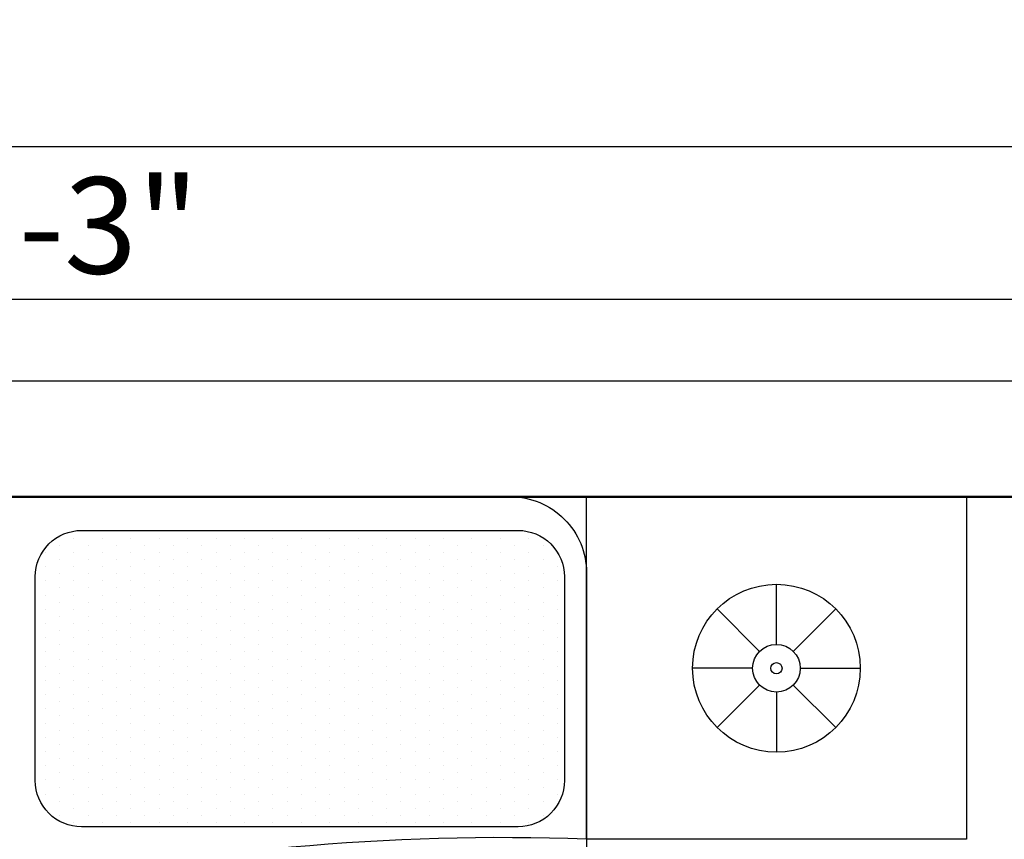
# Model space of a CAD drawing. Units: inches. Extents: x 3064 to 19385, y 846 to 15425.
# Tile 63 of 108: x 6281 to 6332, y 1964 to 2007. Entities that reach past the tile are written whole.
import ezdxf

# ---------------------------------------------------------------- set-up
doc = ezdxf.new("R2010")
doc.units = ezdxf.units.IN
for name, color, linetype, lineweight in [('A-ANNO-DIMS', 2, 'Continuous', 18), ('A-FLOR-FIXT', 9, 'Continuous', 18), ('A-WALL', 7, 'Continuous', 50), ('C-PROP', 6, 'Continuous', 25)]:
    doc.layers.add(name, color=color, linetype=linetype, lineweight=lineweight)
doc.layers.add('BLOCK', color=6, linetype='Continuous')
doc.styles.get("Standard").update_dxf_attribs({"font": 'arial.ttf'})
doc.dimstyles.new('ISO-25', dxfattribs={"dimtxt": 9, "dimasz": 2.5, "dimexe": 1.25, "dimexo": 0.625, "dimtad": 1, "dimdec": 1, "dimlunit": 3, "dimtxsty": 'Standard', "dimcen": 2.5, "dimadec": 0, "dimazin": 0, "dimtfac": 1, "dimtdec": 1, "dimtmove": 0, "dimatfit": 3, "dimfxl": 1, "dimarcsym": 0})

# ---------------------------------------------------------------- blocks, each defined once
blk = doc.blocks.new('*X7')
at = {"color": 0}
for p, q in [((273.75, 456.9375), (273.75, 456.9375)), ((273.9375, 457.03125), (273.9375, 457.03125)), ((274.125, 456.9375), (274.125, 456.9375)), ((274.3125, 457.03125), (274.3125, 457.03125)), ((274.5, 456.9375), (274.5, 456.9375)), ((274.6875, 457.03125), (274.6875, 457.03125)), ((274.875, 456.9375), (274.875, 456.9375)), ((275.0625, 457.03125), (275.0625, 457.03125)), ((275.25, 456.9375), (275.25, 456.9375)), ((275.4375, 457.03125), (275.4375, 457.03125)), ((275.625, 456.9375), (275.625, 456.9375)), ((275.8125, 457.03125), (275.8125, 457.03125)), ((276, 456.9375), (276, 456.9375)), ((276.1875, 457.03125), (276.1875, 457.03125)), ((276.375, 456.9375), (276.375, 456.9375)), ((276.5625, 457.03125), (276.5625, 457.03125)), ((276.75, 456.9375), (276.75, 456.9375)), ((276.9375, 457.03125), (276.9375, 457.03125)), ((277.125, 456.9375), (277.125, 456.9375)), ((277.3125, 457.03125), (277.3125, 457.03125)), ((277.5, 456.9375), (277.5, 456.9375)), ((277.6875, 457.03125), (277.6875, 457.03125)), ((277.875, 456.9375), (277.875, 456.9375)), ((278.0625, 457.03125), (278.0625, 457.03125)), ((278.25, 456.9375), (278.25, 456.9375)), ((278.4375, 457.03125), (278.4375, 457.03125)), ((278.625, 456.9375), (278.625, 456.9375)), ((278.8125, 457.03125), (278.8125, 457.03125)), ((279, 456.9375), (279, 456.9375)), ((279.1875, 457.03125), (279.1875, 457.03125)), ((279.375, 456.9375), (279.375, 456.9375)), ((279.5625, 457.03125), (279.5625, 457.03125)), ((279.75, 456.9375), (279.75, 456.9375)), ((273.5625, 456.84375), (273.5625, 456.84375)), ((273.9375, 456.84375), (273.9375, 456.84375)), ((274.3125, 456.84375), (274.3125, 456.84375)), ((274.6875, 456.84375), (274.6875, 456.84375)), ((275.0625, 456.84375), (275.0625, 456.84375)), ((275.4375, 456.84375), (275.4375, 456.84375)), ((275.8125, 456.84375), (275.8125, 456.84375)), ((276.1875, 456.84375), (276.1875, 456.84375)), ((276.5625, 456.84375), (276.5625, 456.84375)), ((276.9375, 456.84375), (276.9375, 456.84375)), ((277.3125, 456.84375), (277.3125, 456.84375)), ((277.6875, 456.84375), (277.6875, 456.84375)), ((278.0625, 456.84375), (278.0625, 456.84375)), ((278.4375, 456.84375), (278.4375, 456.84375)), ((278.8125, 456.84375), (278.8125, 456.84375)), ((279.1875, 456.84375), (279.1875, 456.84375)), ((279.5625, 456.84375), (279.5625, 456.84375)), ((279.9375, 456.84375), (279.9375, 456.84375)), ((273.375, 456.75), (273.375, 456.75)), ((273.5625, 456.65625), (273.5625, 456.65625)), ((273.75, 456.75), (273.75, 456.75)), ((273.9375, 456.65625), (273.9375, 456.65625)), ((274.125, 456.75), (274.125, 456.75)), ((274.3125, 456.65625), (274.3125, 456.65625)), ((274.5, 456.75), (274.5, 456.75)), ((274.6875, 456.65625), (274.6875, 456.65625)), ((274.875, 456.75), (274.875, 456.75)), ((275.0625, 456.65625), (275.0625, 456.65625)), ((275.25, 456.75), (275.25, 456.75)), ((275.4375, 456.65625), (275.4375, 456.65625)), ((275.625, 456.75), (275.625, 456.75)), ((275.8125, 456.65625), (275.8125, 456.65625)), ((276, 456.75), (276, 456.75)), ((276.1875, 456.65625), (276.1875, 456.65625)), ((276.375, 456.75), (276.375, 456.75)), ((276.5625, 456.65625), (276.5625, 456.65625)), ((276.75, 456.75), (276.75, 456.75)), ((276.9375, 456.65625), (276.9375, 456.65625)), ((277.125, 456.75), (277.125, 456.75)), ((277.3125, 456.65625), (277.3125, 456.65625)), ((277.5, 456.75), (277.5, 456.75)), ((277.6875, 456.65625), (277.6875, 456.65625)), ((277.875, 456.75), (277.875, 456.75)), ((278.0625, 456.65625), (278.0625, 456.65625)), ((278.25, 456.75), (278.25, 456.75)), ((278.4375, 456.65625), (278.4375, 456.65625)), ((278.625, 456.75), (278.625, 456.75)), ((278.8125, 456.65625), (278.8125, 456.65625)), ((279, 456.75), (279, 456.75)), ((279.1875, 456.65625), (279.1875, 456.65625)), ((279.375, 456.75), (279.375, 456.75)), ((279.5625, 456.65625), (279.5625, 456.65625)), ((279.75, 456.75), (279.75, 456.75)), ((279.9375, 456.65625), (279.9375, 456.65625)), ((280.125, 456.75), (280.125, 456.75)), ((273.375, 456.5625), (273.375, 456.5625)), ((273.75, 456.5625), (273.75, 456.5625)), ((274.125, 456.5625), (274.125, 456.5625)), ((274.5, 456.5625), (274.5, 456.5625)), ((274.875, 456.5625), (274.875, 456.5625)), ((275.25, 456.5625), (275.25, 456.5625)), ((275.625, 456.5625), (275.625, 456.5625)), ((276, 456.5625), (276, 456.5625)), ((276.375, 456.5625), (276.375, 456.5625)), ((276.75, 456.5625), (276.75, 456.5625)), ((277.125, 456.5625), (277.125, 456.5625)), ((277.5, 456.5625), (277.5, 456.5625)), ((277.875, 456.5625), (277.875, 456.5625)), ((278.25, 456.5625), (278.25, 456.5625)), ((278.625, 456.5625), (278.625, 456.5625)), ((279, 456.5625), (279, 456.5625)), ((279.375, 456.5625), (279.375, 456.5625)), ((279.75, 456.5625), (279.75, 456.5625)), ((280.125, 456.5625), (280.125, 456.5625)), ((273.5625, 456.46875), (273.5625, 456.46875)), ((273.9375, 456.46875), (273.9375, 456.46875)), ((274.3125, 456.46875), (274.3125, 456.46875)), ((274.6875, 456.46875), (274.6875, 456.46875)), ((275.0625, 456.46875), (275.0625, 456.46875)), ((275.4375, 456.46875), (275.4375, 456.46875)), ((275.8125, 456.46875), (275.8125, 456.46875)), ((276.1875, 456.46875), (276.1875, 456.46875)), ((276.5625, 456.46875), (276.5625, 456.46875)), ((276.9375, 456.46875), (276.9375, 456.46875)), ((277.3125, 456.46875), (277.3125, 456.46875)), ((277.6875, 456.46875), (277.6875, 456.46875)), ((278.0625, 456.46875), (278.0625, 456.46875)), ((278.4375, 456.46875), (278.4375, 456.46875)), ((278.8125, 456.46875), (278.8125, 456.46875)), ((279.1875, 456.46875), (279.1875, 456.46875)), ((279.5625, 456.46875), (279.5625, 456.46875)), ((279.9375, 456.46875), (279.9375, 456.46875)), ((273.375, 456.375), (273.375, 456.375)), ((273.5625, 456.28125), (273.5625, 456.28125)), ((273.75, 456.375), (273.75, 456.375)), ((273.9375, 456.28125), (273.9375, 456.28125)), ((274.125, 456.375), (274.125, 456.375)), ((274.3125, 456.28125), (274.3125, 456.28125)), ((274.5, 456.375), (274.5, 456.375)), ((274.6875, 456.28125), (274.6875, 456.28125)), ((274.875, 456.375), (274.875, 456.375)), ((275.0625, 456.28125), (275.0625, 456.28125)), ((275.25, 456.375), (275.25, 456.375)), ((275.4375, 456.28125), (275.4375, 456.28125)), ((275.625, 456.375), (275.625, 456.375)), ((275.8125, 456.28125), (275.8125, 456.28125)), ((276, 456.375), (276, 456.375)), ((276.1875, 456.28125), (276.1875, 456.28125)), ((276.375, 456.375), (276.375, 456.375)), ((276.5625, 456.28125), (276.5625, 456.28125)), ((276.75, 456.375), (276.75, 456.375)), ((276.9375, 456.28125), (276.9375, 456.28125)), ((277.125, 456.375), (277.125, 456.375)), ((277.3125, 456.28125), (277.3125, 456.28125)), ((277.5, 456.375), (277.5, 456.375)), ((277.6875, 456.28125), (277.6875, 456.28125)), ((277.875, 456.375), (277.875, 456.375)), ((278.0625, 456.28125), (278.0625, 456.28125)), ((278.25, 456.375), (278.25, 456.375)), ((278.4375, 456.28125), (278.4375, 456.28125)), ((278.625, 456.375), (278.625, 456.375)), ((278.8125, 456.28125), (278.8125, 456.28125)), ((279, 456.375), (279, 456.375)), ((279.1875, 456.28125), (279.1875, 456.28125)), ((279.375, 456.375), (279.375, 456.375)), ((279.5625, 456.28125), (279.5625, 456.28125)), ((279.75, 456.375), (279.75, 456.375)), ((279.9375, 456.28125), (279.9375, 456.28125)), ((280.125, 456.375), (280.125, 456.375)), ((273.375, 456.1875), (273.375, 456.1875)), ((273.75, 456.1875), (273.75, 456.1875)), ((274.125, 456.1875), (274.125, 456.1875)), ((274.5, 456.1875), (274.5, 456.1875)), ((274.875, 456.1875), (274.875, 456.1875)), ((275.25, 456.1875), (275.25, 456.1875)), ((275.625, 456.1875), (275.625, 456.1875)), ((276, 456.1875), (276, 456.1875)), ((276.375, 456.1875), (276.375, 456.1875)), ((276.75, 456.1875), (276.75, 456.1875)), ((277.125, 456.1875), (277.125, 456.1875)), ((277.5, 456.1875), (277.5, 456.1875)), ((277.875, 456.1875), (277.875, 456.1875)), ((278.25, 456.1875), (278.25, 456.1875)), ((278.625, 456.1875), (278.625, 456.1875)), ((279, 456.1875), (279, 456.1875)), ((279.375, 456.1875), (279.375, 456.1875)), ((279.75, 456.1875), (279.75, 456.1875)), ((280.125, 456.1875), (280.125, 456.1875)), ((273.375, 456), (273.375, 456)), ((273.5625, 456.09375), (273.5625, 456.09375)), ((273.75, 456), (273.75, 456)), ((273.9375, 456.09375), (273.9375, 456.09375)), ((274.125, 456), (274.125, 456)), ((274.3125, 456.09375), (274.3125, 456.09375)), ((274.5, 456), (274.5, 456)), ((274.6875, 456.09375), (274.6875, 456.09375)), ((274.875, 456), (274.875, 456)), ((275.0625, 456.09375), (275.0625, 456.09375)), ((275.25, 456), (275.25, 456)), ((275.4375, 456.09375), (275.4375, 456.09375)), ((275.625, 456), (275.625, 456)), ((275.8125, 456.09375), (275.8125, 456.09375)), ((276, 456), (276, 456)), ((276.1875, 456.09375), (276.1875, 456.09375)), ((276.375, 456), (276.375, 456)), ((276.5625, 456.09375), (276.5625, 456.09375)), ((276.75, 456), (276.75, 456)), ((276.9375, 456.09375), (276.9375, 456.09375)), ((277.125, 456), (277.125, 456)), ((277.3125, 456.09375), (277.3125, 456.09375)), ((277.5, 456), (277.5, 456)), ((277.6875, 456.09375), (277.6875, 456.09375)), ((277.875, 456), (277.875, 456)), ((278.0625, 456.09375), (278.0625, 456.09375)), ((278.25, 456), (278.25, 456)), ((278.4375, 456.09375), (278.4375, 456.09375)), ((278.625, 456), (278.625, 456)), ((278.8125, 456.09375), (278.8125, 456.09375)), ((279, 456), (279, 456)), ((279.1875, 456.09375), (279.1875, 456.09375)), ((279.375, 456), (279.375, 456)), ((279.5625, 456.09375), (279.5625, 456.09375)), ((279.75, 456), (279.75, 456)), ((279.9375, 456.09375), (279.9375, 456.09375)), ((280.125, 456), (280.125, 456)), ((273.5625, 455.90625), (273.5625, 455.90625)), ((273.9375, 455.90625), (273.9375, 455.90625)), ((274.3125, 455.90625), (274.3125, 455.90625)), ((274.6875, 455.90625), (274.6875, 455.90625)), ((275.0625, 455.90625), (275.0625, 455.90625)), ((275.4375, 455.90625), (275.4375, 455.90625)), ((275.8125, 455.90625), (275.8125, 455.90625)), ((276.1875, 455.90625), (276.1875, 455.90625)), ((276.5625, 455.90625), (276.5625, 455.90625)), ((276.9375, 455.90625), (276.9375, 455.90625)), ((277.3125, 455.90625), (277.3125, 455.90625)), ((277.6875, 455.90625), (277.6875, 455.90625)), ((278.0625, 455.90625), (278.0625, 455.90625)), ((278.4375, 455.90625), (278.4375, 455.90625)), ((278.8125, 455.90625), (278.8125, 455.90625)), ((279.1875, 455.90625), (279.1875, 455.90625)), ((279.5625, 455.90625), (279.5625, 455.90625)), ((279.9375, 455.90625), (279.9375, 455.90625)), ((273.375, 455.8125), (273.375, 455.8125)), ((273.75, 455.8125), (273.75, 455.8125)), ((274.125, 455.8125), (274.125, 455.8125)), ((274.5, 455.8125), (274.5, 455.8125)), ((274.875, 455.8125), (274.875, 455.8125)), ((275.25, 455.8125), (275.25, 455.8125)), ((275.625, 455.8125), (275.625, 455.8125)), ((276, 455.8125), (276, 455.8125)), ((276.375, 455.8125), (276.375, 455.8125)), ((276.75, 455.8125), (276.75, 455.8125)), ((277.125, 455.8125), (277.125, 455.8125)), ((277.5, 455.8125), (277.5, 455.8125)), ((277.875, 455.8125), (277.875, 455.8125)), ((278.25, 455.8125), (278.25, 455.8125)), ((278.625, 455.8125), (278.625, 455.8125)), ((279, 455.8125), (279, 455.8125)), ((279.375, 455.8125), (279.375, 455.8125)), ((279.75, 455.8125), (279.75, 455.8125)), ((280.125, 455.8125), (280.125, 455.8125)), ((273.375, 455.625), (273.375, 455.625)), ((273.5625, 455.71875), (273.5625, 455.71875)), ((273.75, 455.625), (273.75, 455.625)), ((273.9375, 455.71875), (273.9375, 455.71875)), ((274.125, 455.625), (274.125, 455.625)), ((274.3125, 455.71875), (274.3125, 455.71875)), ((274.5, 455.625), (274.5, 455.625)), ((274.6875, 455.71875), (274.6875, 455.71875)), ((274.875, 455.625), (274.875, 455.625)), ((275.0625, 455.71875), (275.0625, 455.71875)), ((275.25, 455.625), (275.25, 455.625)), ((275.4375, 455.71875), (275.4375, 455.71875)), ((275.625, 455.625), (275.625, 455.625)), ((275.8125, 455.71875), (275.8125, 455.71875)), ((276, 455.625), (276, 455.625)), ((276.1875, 455.71875), (276.1875, 455.71875)), ((276.375, 455.625), (276.375, 455.625)), ((276.5625, 455.71875), (276.5625, 455.71875)), ((276.75, 455.625), (276.75, 455.625)), ((276.9375, 455.71875), (276.9375, 455.71875)), ((277.125, 455.625), (277.125, 455.625)), ((277.3125, 455.71875), (277.3125, 455.71875)), ((277.5, 455.625), (277.5, 455.625)), ((277.6875, 455.71875), (277.6875, 455.71875)), ((277.875, 455.625), (277.875, 455.625)), ((278.0625, 455.71875), (278.0625, 455.71875)), ((278.25, 455.625), (278.25, 455.625)), ((278.4375, 455.71875), (278.4375, 455.71875)), ((278.625, 455.625), (278.625, 455.625)), ((278.8125, 455.71875), (278.8125, 455.71875)), ((279, 455.625), (279, 455.625)), ((279.1875, 455.71875), (279.1875, 455.71875)), ((279.375, 455.625), (279.375, 455.625)), ((279.5625, 455.71875), (279.5625, 455.71875)), ((279.75, 455.625), (279.75, 455.625)), ((279.9375, 455.71875), (279.9375, 455.71875)), ((280.125, 455.625), (280.125, 455.625)), ((273.5625, 455.53125), (273.5625, 455.53125)), ((273.9375, 455.53125), (273.9375, 455.53125)), ((274.3125, 455.53125), (274.3125, 455.53125)), ((274.6875, 455.53125), (274.6875, 455.53125)), ((275.0625, 455.53125), (275.0625, 455.53125)), ((275.4375, 455.53125), (275.4375, 455.53125)), ((275.8125, 455.53125), (275.8125, 455.53125)), ((276.1875, 455.53125), (276.1875, 455.53125)), ((276.5625, 455.53125), (276.5625, 455.53125)), ((276.9375, 455.53125), (276.9375, 455.53125)), ((277.3125, 455.53125), (277.3125, 455.53125)), ((277.6875, 455.53125), (277.6875, 455.53125)), ((278.0625, 455.53125), (278.0625, 455.53125)), ((278.4375, 455.53125), (278.4375, 455.53125)), ((278.8125, 455.53125), (278.8125, 455.53125)), ((279.1875, 455.53125), (279.1875, 455.53125)), ((279.5625, 455.53125), (279.5625, 455.53125)), ((279.9375, 455.53125), (279.9375, 455.53125)), ((273.375, 455.4375), (273.375, 455.4375)), ((273.75, 455.4375), (273.75, 455.4375)), ((274.125, 455.4375), (274.125, 455.4375)), ((274.5, 455.4375), (274.5, 455.4375)), ((274.875, 455.4375), (274.875, 455.4375)), ((275.25, 455.4375), (275.25, 455.4375)), ((275.625, 455.4375), (275.625, 455.4375)), ((276, 455.4375), (276, 455.4375)), ((276.375, 455.4375), (276.375, 455.4375)), ((276.75, 455.4375), (276.75, 455.4375)), ((277.125, 455.4375), (277.125, 455.4375)), ((277.5, 455.4375), (277.5, 455.4375)), ((277.875, 455.4375), (277.875, 455.4375)), ((278.25, 455.4375), (278.25, 455.4375)), ((278.625, 455.4375), (278.625, 455.4375)), ((279, 455.4375), (279, 455.4375)), ((279.375, 455.4375), (279.375, 455.4375)), ((279.75, 455.4375), (279.75, 455.4375)), ((280.125, 455.4375), (280.125, 455.4375)), ((273.375, 455.25), (273.375, 455.25)), ((273.5625, 455.34375), (273.5625, 455.34375)), ((273.75, 455.25), (273.75, 455.25)), ((273.9375, 455.34375), (273.9375, 455.34375)), ((274.125, 455.25), (274.125, 455.25)), ((274.3125, 455.34375), (274.3125, 455.34375)), ((274.5, 455.25), (274.5, 455.25)), ((274.6875, 455.34375), (274.6875, 455.34375)), ((274.875, 455.25), (274.875, 455.25)), ((275.0625, 455.34375), (275.0625, 455.34375)), ((275.25, 455.25), (275.25, 455.25)), ((275.4375, 455.34375), (275.4375, 455.34375)), ((275.625, 455.25), (275.625, 455.25)), ((275.8125, 455.34375), (275.8125, 455.34375)), ((276, 455.25), (276, 455.25)), ((276.1875, 455.34375), (276.1875, 455.34375)), ((276.375, 455.25), (276.375, 455.25)), ((276.5625, 455.34375), (276.5625, 455.34375)), ((276.75, 455.25), (276.75, 455.25)), ((276.9375, 455.34375), (276.9375, 455.34375)), ((277.125, 455.25), (277.125, 455.25)), ((277.3125, 455.34375), (277.3125, 455.34375)), ((277.5, 455.25), (277.5, 455.25)), ((277.6875, 455.34375), (277.6875, 455.34375)), ((277.875, 455.25), (277.875, 455.25)), ((278.0625, 455.34375), (278.0625, 455.34375)), ((278.25, 455.25), (278.25, 455.25)), ((278.4375, 455.34375), (278.4375, 455.34375)), ((278.625, 455.25), (278.625, 455.25)), ((278.8125, 455.34375), (278.8125, 455.34375)), ((279, 455.25), (279, 455.25)), ((279.1875, 455.34375), (279.1875, 455.34375)), ((279.375, 455.25), (279.375, 455.25)), ((279.5625, 455.34375), (279.5625, 455.34375)), ((279.75, 455.25), (279.75, 455.25)), ((279.9375, 455.34375), (279.9375, 455.34375)), ((280.125, 455.25), (280.125, 455.25)), ((273.5625, 455.15625), (273.5625, 455.15625)), ((273.9375, 455.15625), (273.9375, 455.15625)), ((274.3125, 455.15625), (274.3125, 455.15625)), ((274.6875, 455.15625), (274.6875, 455.15625)), ((275.0625, 455.15625), (275.0625, 455.15625)), ((275.4375, 455.15625), (275.4375, 455.15625)), ((275.8125, 455.15625), (275.8125, 455.15625)), ((276.1875, 455.15625), (276.1875, 455.15625)), ((276.5625, 455.15625), (276.5625, 455.15625)), ((276.9375, 455.15625), (276.9375, 455.15625)), ((277.3125, 455.15625), (277.3125, 455.15625)), ((277.6875, 455.15625), (277.6875, 455.15625)), ((278.0625, 455.15625), (278.0625, 455.15625)), ((278.4375, 455.15625), (278.4375, 455.15625)), ((278.8125, 455.15625), (278.8125, 455.15625)), ((279.1875, 455.15625), (279.1875, 455.15625)), ((279.5625, 455.15625), (279.5625, 455.15625)), ((279.9375, 455.15625), (279.9375, 455.15625)), ((273.375, 455.0625), (273.375, 455.0625)), ((273.5625, 454.96875), (273.5625, 454.96875)), ((273.75, 455.0625), (273.75, 455.0625)), ((273.9375, 454.96875), (273.9375, 454.96875)), ((274.125, 455.0625), (274.125, 455.0625)), ((274.3125, 454.96875), (274.3125, 454.96875)), ((274.5, 455.0625), (274.5, 455.0625)), ((274.6875, 454.96875), (274.6875, 454.96875)), ((274.875, 455.0625), (274.875, 455.0625)), ((275.0625, 454.96875), (275.0625, 454.96875)), ((275.25, 455.0625), (275.25, 455.0625)), ((275.4375, 454.96875), (275.4375, 454.96875)), ((275.625, 455.0625), (275.625, 455.0625)), ((275.8125, 454.96875), (275.8125, 454.96875)), ((276, 455.0625), (276, 455.0625)), ((276.1875, 454.96875), (276.1875, 454.96875)), ((276.375, 455.0625), (276.375, 455.0625)), ((276.5625, 454.96875), (276.5625, 454.96875)), ((276.75, 455.0625), (276.75, 455.0625)), ((276.9375, 454.96875), (276.9375, 454.96875)), ((277.125, 455.0625), (277.125, 455.0625)), ((277.3125, 454.96875), (277.3125, 454.96875)), ((277.5, 455.0625), (277.5, 455.0625)), ((277.6875, 454.96875), (277.6875, 454.96875)), ((277.875, 455.0625), (277.875, 455.0625)), ((278.0625, 454.96875), (278.0625, 454.96875)), ((278.25, 455.0625), (278.25, 455.0625)), ((278.4375, 454.96875), (278.4375, 454.96875)), ((278.625, 455.0625), (278.625, 455.0625)), ((278.8125, 454.96875), (278.8125, 454.96875)), ((279, 455.0625), (279, 455.0625)), ((279.1875, 454.96875), (279.1875, 454.96875)), ((279.375, 455.0625), (279.375, 455.0625)), ((279.5625, 454.96875), (279.5625, 454.96875)), ((279.75, 455.0625), (279.75, 455.0625)), ((279.9375, 454.96875), (279.9375, 454.96875)), ((280.125, 455.0625), (280.125, 455.0625)), ((273.375, 454.875), (273.375, 454.875)), ((273.75, 454.875), (273.75, 454.875)), ((274.125, 454.875), (274.125, 454.875)), ((274.5, 454.875), (274.5, 454.875)), ((274.875, 454.875), (274.875, 454.875)), ((275.25, 454.875), (275.25, 454.875)), ((275.625, 454.875), (275.625, 454.875)), ((276, 454.875), (276, 454.875)), ((276.375, 454.875), (276.375, 454.875)), ((276.75, 454.875), (276.75, 454.875)), ((277.125, 454.875), (277.125, 454.875)), ((277.5, 454.875), (277.5, 454.875)), ((277.875, 454.875), (277.875, 454.875)), ((278.25, 454.875), (278.25, 454.875)), ((278.625, 454.875), (278.625, 454.875)), ((279, 454.875), (279, 454.875)), ((279.375, 454.875), (279.375, 454.875)), ((279.75, 454.875), (279.75, 454.875)), ((280.125, 454.875), (280.125, 454.875)), ((273.5625, 454.78125), (273.5625, 454.78125)), ((273.9375, 454.78125), (273.9375, 454.78125)), ((274.3125, 454.78125), (274.3125, 454.78125)), ((274.6875, 454.78125), (274.6875, 454.78125)), ((275.0625, 454.78125), (275.0625, 454.78125)), ((275.4375, 454.78125), (275.4375, 454.78125)), ((275.8125, 454.78125), (275.8125, 454.78125)), ((276.1875, 454.78125), (276.1875, 454.78125)), ((276.5625, 454.78125), (276.5625, 454.78125)), ((276.9375, 454.78125), (276.9375, 454.78125)), ((277.3125, 454.78125), (277.3125, 454.78125)), ((277.6875, 454.78125), (277.6875, 454.78125)), ((278.0625, 454.78125), (278.0625, 454.78125)), ((278.4375, 454.78125), (278.4375, 454.78125)), ((278.8125, 454.78125), (278.8125, 454.78125)), ((279.1875, 454.78125), (279.1875, 454.78125)), ((279.5625, 454.78125), (279.5625, 454.78125)), ((279.9375, 454.78125), (279.9375, 454.78125)), ((273.375, 454.6875), (273.375, 454.6875)), ((273.5625, 454.59375), (273.5625, 454.59375)), ((273.75, 454.6875), (273.75, 454.6875)), ((273.9375, 454.59375), (273.9375, 454.59375)), ((274.125, 454.6875), (274.125, 454.6875)), ((274.3125, 454.59375), (274.3125, 454.59375)), ((274.5, 454.6875), (274.5, 454.6875)), ((274.6875, 454.59375), (274.6875, 454.59375)), ((274.875, 454.6875), (274.875, 454.6875)), ((275.0625, 454.59375), (275.0625, 454.59375)), ((275.25, 454.6875), (275.25, 454.6875)), ((275.4375, 454.59375), (275.4375, 454.59375)), ((275.625, 454.6875), (275.625, 454.6875)), ((275.8125, 454.59375), (275.8125, 454.59375)), ((276, 454.6875), (276, 454.6875)), ((276.1875, 454.59375), (276.1875, 454.59375)), ((276.375, 454.6875), (276.375, 454.6875)), ((276.5625, 454.59375), (276.5625, 454.59375)), ((276.75, 454.6875), (276.75, 454.6875)), ((276.9375, 454.59375), (276.9375, 454.59375)), ((277.125, 454.6875), (277.125, 454.6875)), ((277.3125, 454.59375), (277.3125, 454.59375)), ((277.5, 454.6875), (277.5, 454.6875)), ((277.6875, 454.59375), (277.6875, 454.59375)), ((277.875, 454.6875), (277.875, 454.6875)), ((278.0625, 454.59375), (278.0625, 454.59375)), ((278.25, 454.6875), (278.25, 454.6875)), ((278.4375, 454.59375), (278.4375, 454.59375)), ((278.625, 454.6875), (278.625, 454.6875)), ((278.8125, 454.59375), (278.8125, 454.59375)), ((279, 454.6875), (279, 454.6875)), ((279.1875, 454.59375), (279.1875, 454.59375)), ((279.375, 454.6875), (279.375, 454.6875)), ((279.5625, 454.59375), (279.5625, 454.59375)), ((279.75, 454.6875), (279.75, 454.6875)), ((279.9375, 454.59375), (279.9375, 454.59375)), ((280.125, 454.6875), (280.125, 454.6875)), ((273.375, 454.5), (273.375, 454.5)), ((273.75, 454.5), (273.75, 454.5)), ((274.125, 454.5), (274.125, 454.5)), ((274.5, 454.5), (274.5, 454.5)), ((274.875, 454.5), (274.875, 454.5)), ((275.25, 454.5), (275.25, 454.5)), ((275.625, 454.5), (275.625, 454.5)), ((276, 454.5), (276, 454.5)), ((276.375, 454.5), (276.375, 454.5)), ((276.75, 454.5), (276.75, 454.5)), ((277.125, 454.5), (277.125, 454.5)), ((277.5, 454.5), (277.5, 454.5)), ((277.875, 454.5), (277.875, 454.5)), ((278.25, 454.5), (278.25, 454.5)), ((278.625, 454.5), (278.625, 454.5)), ((279, 454.5), (279, 454.5)), ((279.375, 454.5), (279.375, 454.5)), ((279.75, 454.5), (279.75, 454.5)), ((280.125, 454.5), (280.125, 454.5)), ((273.375, 454.3125), (273.375, 454.3125)), ((273.5625, 454.40625), (273.5625, 454.40625)), ((273.75, 454.3125), (273.75, 454.3125)), ((273.9375, 454.40625), (273.9375, 454.40625)), ((274.125, 454.3125), (274.125, 454.3125)), ((274.3125, 454.40625), (274.3125, 454.40625)), ((274.5, 454.3125), (274.5, 454.3125)), ((274.6875, 454.40625), (274.6875, 454.40625)), ((274.875, 454.3125), (274.875, 454.3125)), ((275.0625, 454.40625), (275.0625, 454.40625)), ((275.25, 454.3125), (275.25, 454.3125)), ((275.4375, 454.40625), (275.4375, 454.40625)), ((275.625, 454.3125), (275.625, 454.3125)), ((275.8125, 454.40625), (275.8125, 454.40625)), ((276, 454.3125), (276, 454.3125)), ((276.1875, 454.40625), (276.1875, 454.40625)), ((276.375, 454.3125), (276.375, 454.3125)), ((276.5625, 454.40625), (276.5625, 454.40625)), ((276.75, 454.3125), (276.75, 454.3125)), ((276.9375, 454.40625), (276.9375, 454.40625)), ((277.125, 454.3125), (277.125, 454.3125)), ((277.3125, 454.40625), (277.3125, 454.40625)), ((277.5, 454.3125), (277.5, 454.3125)), ((277.6875, 454.40625), (277.6875, 454.40625)), ((277.875, 454.3125), (277.875, 454.3125)), ((278.0625, 454.40625), (278.0625, 454.40625)), ((278.25, 454.3125), (278.25, 454.3125)), ((278.4375, 454.40625), (278.4375, 454.40625)), ((278.625, 454.3125), (278.625, 454.3125)), ((278.8125, 454.40625), (278.8125, 454.40625)), ((279, 454.3125), (279, 454.3125)), ((279.1875, 454.40625), (279.1875, 454.40625)), ((279.375, 454.3125), (279.375, 454.3125)), ((279.5625, 454.40625), (279.5625, 454.40625)), ((279.75, 454.3125), (279.75, 454.3125)), ((279.9375, 454.40625), (279.9375, 454.40625)), ((280.125, 454.3125), (280.125, 454.3125)), ((273.5625, 454.21875), (273.5625, 454.21875)), ((273.9375, 454.21875), (273.9375, 454.21875)), ((274.3125, 454.21875), (274.3125, 454.21875)), ((274.6875, 454.21875), (274.6875, 454.21875)), ((275.0625, 454.21875), (275.0625, 454.21875)), ((275.4375, 454.21875), (275.4375, 454.21875)), ((275.8125, 454.21875), (275.8125, 454.21875)), ((276.1875, 454.21875), (276.1875, 454.21875)), ((276.5625, 454.21875), (276.5625, 454.21875)), ((276.9375, 454.21875), (276.9375, 454.21875)), ((277.3125, 454.21875), (277.3125, 454.21875)), ((277.6875, 454.21875), (277.6875, 454.21875)), ((278.0625, 454.21875), (278.0625, 454.21875)), ((278.4375, 454.21875), (278.4375, 454.21875)), ((278.8125, 454.21875), (278.8125, 454.21875)), ((279.1875, 454.21875), (279.1875, 454.21875)), ((279.5625, 454.21875), (279.5625, 454.21875)), ((279.9375, 454.21875), (279.9375, 454.21875)), ((273.375, 454.125), (273.375, 454.125)), ((273.75, 454.125), (273.75, 454.125)), ((274.125, 454.125), (274.125, 454.125)), ((274.5, 454.125), (274.5, 454.125)), ((274.875, 454.125), (274.875, 454.125)), ((275.25, 454.125), (275.25, 454.125)), ((275.625, 454.125), (275.625, 454.125)), ((276, 454.125), (276, 454.125)), ((276.375, 454.125), (276.375, 454.125)), ((276.75, 454.125), (276.75, 454.125)), ((277.125, 454.125), (277.125, 454.125)), ((277.5, 454.125), (277.5, 454.125)), ((277.875, 454.125), (277.875, 454.125)), ((278.25, 454.125), (278.25, 454.125)), ((278.625, 454.125), (278.625, 454.125)), ((279, 454.125), (279, 454.125)), ((279.375, 454.125), (279.375, 454.125)), ((279.75, 454.125), (279.75, 454.125)), ((280.125, 454.125), (280.125, 454.125)), ((273.375, 453.9375), (273.375, 453.9375)), ((273.5625, 454.03125), (273.5625, 454.03125)), ((273.75, 453.9375), (273.75, 453.9375)), ((273.9375, 454.03125), (273.9375, 454.03125)), ((274.125, 453.9375), (274.125, 453.9375)), ((274.3125, 454.03125), (274.3125, 454.03125)), ((274.5, 453.9375), (274.5, 453.9375)), ((274.6875, 454.03125), (274.6875, 454.03125)), ((274.875, 453.9375), (274.875, 453.9375)), ((275.0625, 454.03125), (275.0625, 454.03125)), ((275.25, 453.9375), (275.25, 453.9375)), ((275.4375, 454.03125), (275.4375, 454.03125)), ((275.625, 453.9375), (275.625, 453.9375)), ((275.8125, 454.03125), (275.8125, 454.03125)), ((276, 453.9375), (276, 453.9375)), ((276.1875, 454.03125), (276.1875, 454.03125)), ((276.375, 453.9375), (276.375, 453.9375)), ((276.5625, 454.03125), (276.5625, 454.03125)), ((276.75, 453.9375), (276.75, 453.9375)), ((276.9375, 454.03125), (276.9375, 454.03125)), ((277.125, 453.9375), (277.125, 453.9375)), ((277.3125, 454.03125), (277.3125, 454.03125)), ((277.5, 453.9375), (277.5, 453.9375)), ((277.6875, 454.03125), (277.6875, 454.03125)), ((277.875, 453.9375), (277.875, 453.9375)), ((278.0625, 454.03125), (278.0625, 454.03125)), ((278.25, 453.9375), (278.25, 453.9375)), ((278.4375, 454.03125), (278.4375, 454.03125)), ((278.625, 453.9375), (278.625, 453.9375)), ((278.8125, 454.03125), (278.8125, 454.03125)), ((279, 453.9375), (279, 453.9375)), ((279.1875, 454.03125), (279.1875, 454.03125)), ((279.375, 453.9375), (279.375, 453.9375)), ((279.5625, 454.03125), (279.5625, 454.03125)), ((279.75, 453.9375), (279.75, 453.9375)), ((279.9375, 454.03125), (279.9375, 454.03125)), ((280.125, 453.9375), (280.125, 453.9375)), ((273.5625, 453.84375), (273.5625, 453.84375)), ((273.9375, 453.84375), (273.9375, 453.84375)), ((274.3125, 453.84375), (274.3125, 453.84375)), ((274.6875, 453.84375), (274.6875, 453.84375)), ((275.0625, 453.84375), (275.0625, 453.84375)), ((275.4375, 453.84375), (275.4375, 453.84375)), ((275.8125, 453.84375), (275.8125, 453.84375)), ((276.1875, 453.84375), (276.1875, 453.84375)), ((276.5625, 453.84375), (276.5625, 453.84375)), ((276.9375, 453.84375), (276.9375, 453.84375)), ((277.3125, 453.84375), (277.3125, 453.84375)), ((277.6875, 453.84375), (277.6875, 453.84375)), ((278.0625, 453.84375), (278.0625, 453.84375)), ((278.4375, 453.84375), (278.4375, 453.84375)), ((278.8125, 453.84375), (278.8125, 453.84375)), ((279.1875, 453.84375), (279.1875, 453.84375)), ((279.5625, 453.84375), (279.5625, 453.84375)), ((279.9375, 453.84375), (279.9375, 453.84375)), ((273.375, 453.75), (273.375, 453.75)), ((273.75, 453.75), (273.75, 453.75)), ((274.125, 453.75), (274.125, 453.75)), ((274.5, 453.75), (274.5, 453.75)), ((274.875, 453.75), (274.875, 453.75)), ((275.25, 453.75), (275.25, 453.75)), ((275.625, 453.75), (275.625, 453.75)), ((276, 453.75), (276, 453.75)), ((276.375, 453.75), (276.375, 453.75)), ((276.75, 453.75), (276.75, 453.75)), ((277.125, 453.75), (277.125, 453.75)), ((277.5, 453.75), (277.5, 453.75)), ((277.875, 453.75), (277.875, 453.75)), ((278.25, 453.75), (278.25, 453.75)), ((278.625, 453.75), (278.625, 453.75)), ((279, 453.75), (279, 453.75)), ((279.375, 453.75), (279.375, 453.75)), ((279.75, 453.75), (279.75, 453.75)), ((280.125, 453.75), (280.125, 453.75)), ((273.375, 453.5625), (273.375, 453.5625)), ((273.5625, 453.65625), (273.5625, 453.65625)), ((273.75, 453.5625), (273.75, 453.5625)), ((273.9375, 453.65625), (273.9375, 453.65625)), ((274.125, 453.5625), (274.125, 453.5625)), ((274.3125, 453.65625), (274.3125, 453.65625)), ((274.5, 453.5625), (274.5, 453.5625)), ((274.6875, 453.65625), (274.6875, 453.65625)), ((274.875, 453.5625), (274.875, 453.5625)), ((275.0625, 453.65625), (275.0625, 453.65625)), ((275.25, 453.5625), (275.25, 453.5625)), ((275.4375, 453.65625), (275.4375, 453.65625)), ((275.625, 453.5625), (275.625, 453.5625)), ((275.8125, 453.65625), (275.8125, 453.65625)), ((276, 453.5625), (276, 453.5625)), ((276.1875, 453.65625), (276.1875, 453.65625)), ((276.375, 453.5625), (276.375, 453.5625)), ((276.5625, 453.65625), (276.5625, 453.65625)), ((276.75, 453.5625), (276.75, 453.5625)), ((276.9375, 453.65625), (276.9375, 453.65625)), ((277.125, 453.5625), (277.125, 453.5625)), ((277.3125, 453.65625), (277.3125, 453.65625)), ((277.5, 453.5625), (277.5, 453.5625)), ((277.6875, 453.65625), (277.6875, 453.65625)), ((277.875, 453.5625), (277.875, 453.5625)), ((278.0625, 453.65625), (278.0625, 453.65625)), ((278.25, 453.5625), (278.25, 453.5625)), ((278.4375, 453.65625), (278.4375, 453.65625)), ((278.625, 453.5625), (278.625, 453.5625)), ((278.8125, 453.65625), (278.8125, 453.65625)), ((279, 453.5625), (279, 453.5625)), ((279.1875, 453.65625), (279.1875, 453.65625)), ((279.375, 453.5625), (279.375, 453.5625)), ((279.5625, 453.65625), (279.5625, 453.65625)), ((279.75, 453.5625), (279.75, 453.5625)), ((279.9375, 453.65625), (279.9375, 453.65625)), ((280.125, 453.5625), (280.125, 453.5625)), ((273.5625, 453.46875), (273.5625, 453.46875)), ((273.9375, 453.46875), (273.9375, 453.46875)), ((274.3125, 453.46875), (274.3125, 453.46875)), ((274.6875, 453.46875), (274.6875, 453.46875)), ((275.0625, 453.46875), (275.0625, 453.46875)), ((275.4375, 453.46875), (275.4375, 453.46875)), ((275.8125, 453.46875), (275.8125, 453.46875)), ((276.1875, 453.46875), (276.1875, 453.46875)), ((276.5625, 453.46875), (276.5625, 453.46875)), ((276.9375, 453.46875), (276.9375, 453.46875)), ((277.3125, 453.46875), (277.3125, 453.46875)), ((277.6875, 453.46875), (277.6875, 453.46875)), ((278.0625, 453.46875), (278.0625, 453.46875)), ((278.4375, 453.46875), (278.4375, 453.46875)), ((278.8125, 453.46875), (278.8125, 453.46875)), ((279.1875, 453.46875), (279.1875, 453.46875)), ((279.5625, 453.46875), (279.5625, 453.46875)), ((279.9375, 453.46875), (279.9375, 453.46875)), ((273.375, 453.375), (273.375, 453.375)), ((273.5625, 453.28125), (273.5625, 453.28125)), ((273.75, 453.375), (273.75, 453.375)), ((273.9375, 453.28125), (273.9375, 453.28125)), ((274.125, 453.375), (274.125, 453.375)), ((274.3125, 453.28125), (274.3125, 453.28125)), ((274.5, 453.375), (274.5, 453.375)), ((274.6875, 453.28125), (274.6875, 453.28125)), ((274.875, 453.375), (274.875, 453.375)), ((275.0625, 453.28125), (275.0625, 453.28125)), ((275.25, 453.375), (275.25, 453.375)), ((275.4375, 453.28125), (275.4375, 453.28125)), ((275.625, 453.375), (275.625, 453.375)), ((275.8125, 453.28125), (275.8125, 453.28125)), ((276, 453.375), (276, 453.375)), ((276.1875, 453.28125), (276.1875, 453.28125)), ((276.375, 453.375), (276.375, 453.375)), ((276.5625, 453.28125), (276.5625, 453.28125)), ((276.75, 453.375), (276.75, 453.375)), ((276.9375, 453.28125), (276.9375, 453.28125)), ((277.125, 453.375), (277.125, 453.375)), ((277.3125, 453.28125), (277.3125, 453.28125)), ((277.5, 453.375), (277.5, 453.375)), ((277.6875, 453.28125), (277.6875, 453.28125)), ((277.875, 453.375), (277.875, 453.375)), ((278.0625, 453.28125), (278.0625, 453.28125)), ((278.25, 453.375), (278.25, 453.375)), ((278.4375, 453.28125), (278.4375, 453.28125)), ((278.625, 453.375), (278.625, 453.375)), ((278.8125, 453.28125), (278.8125, 453.28125)), ((279, 453.375), (279, 453.375)), ((279.1875, 453.28125), (279.1875, 453.28125)), ((279.375, 453.375), (279.375, 453.375)), ((279.5625, 453.28125), (279.5625, 453.28125)), ((279.75, 453.375), (279.75, 453.375)), ((279.9375, 453.28125), (279.9375, 453.28125)), ((273.75, 453.1875), (273.75, 453.1875)), ((274.125, 453.1875), (274.125, 453.1875)), ((274.5, 453.1875), (274.5, 453.1875)), ((274.875, 453.1875), (274.875, 453.1875)), ((275.25, 453.1875), (275.25, 453.1875)), ((275.625, 453.1875), (275.625, 453.1875)), ((276, 453.1875), (276, 453.1875)), ((276.375, 453.1875), (276.375, 453.1875)), ((276.75, 453.1875), (276.75, 453.1875)), ((277.125, 453.1875), (277.125, 453.1875)), ((277.5, 453.1875), (277.5, 453.1875)), ((277.875, 453.1875), (277.875, 453.1875)), ((278.25, 453.1875), (278.25, 453.1875)), ((278.625, 453.1875), (278.625, 453.1875)), ((279, 453.1875), (279, 453.1875)), ((279.375, 453.1875), (279.375, 453.1875)), ((279.75, 453.1875), (279.75, 453.1875))]:
    blk.add_line(p, q, dxfattribs=at)
blk = doc.blocks.new('A$C52E67D0D')
at = {"layer": 'BLOCK'}
for p, q in [((2251.5, 1605.5), (2251.5, 1684.7)), ((2229.3, 1596.3), (2173.3, 1652.3)), ((2273.7, 1596.3), (2329.7, 1652.3)), ((2220.1, 1574.1), (2140.9, 1574.1)), ((2282.9, 1574.1), (2362.1, 1574.1)), ((2229.3, 1551.9), (2173.3, 1495.9)), ((2273.7, 1551.9), (2329.7, 1495.9)), ((2251.5, 1542.8), (2251.5, 1463.5))]:
    blk.add_line(p, q, dxfattribs=at)
for points in [[(1901, 0), (601, 0, -0.414214), (501, 100), (501, 1700, -0.414214), (601, 1800), (1901, 1800, -0.414214), (2001, 1700), (2001, 100, -0.414214)], [(1911, 1365.1), (1335, 1365.1, -0.414214), (1274.2, 1425.9), (1274.2, 1694.8, -0.414214), (1335, 1755.7), (1911, 1755.7, -0.414214), (1971.8, 1694.8), (1971.8, 1425.9, -0.414214)]]:
    blk.add_lwpolyline(points, format="xyb", close=True, dxfattribs=at)
blk.add_lwpolyline([(2001, 1348.6), (2001, 1799.6), (2502, 1799.6), (2502, 1348.6)], close=True, dxfattribs=at)
for radius in [110.6, 31.4, 7.46]:
    blk.add_circle((2251.5, 1574.1), radius, dxfattribs=at)
blk.add_arc((1888.6, -1664.5), 3015.3, 87.8642, 117.4001, dxfattribs=at)
at = {"layer": 'BLOCK', "xscale": 100, "yscale": 100, "zscale": 100}
blk.add_blockref('*X7', (-26050, -43948.2), dxfattribs=at)
blk = doc.blocks.new('*D387')
at = {"layer": 'A-ANNO-DIMS', "color": 0, "lineweight": -2, "transparency": 16777216}
for p, q in [((6183.493, 1988.614), (6183.493, 1993.494)), ((6378.493, 1988.614), (6378.493, 1993.494)), ((6185.993, 1992.244), (6375.993, 1992.244))]:
    blk.add_line(p, q, dxfattribs=at)
at = {"layer": 'A-ANNO-DIMS', "color": 0, "transparency": 16777216}
for points in [[(6185.993, 1992.66), (6185.993, 1991.827), (6183.493, 1992.244)], [(6375.993, 1992.66), (6375.993, 1991.827), (6378.493, 1992.244)]]:
    blk.add_solid(points, dxfattribs=at)
at = {"layer": 'Defpoints', "color": 0, "transparency": 16777216}
for p in [(6378.493, 1992.244), (6183.493, 1987.989), (6378.493, 1987.989)]:
    blk.add_point(p, dxfattribs=at)
at = {"layer": 'A-ANNO-DIMS', "color": 0, "transparency": 16777216, "insert": (6280.993, 1995.423), "char_height": 5, "attachment_point": 5}
blk.add_mtext('16\'-3"', dxfattribs=at)
blk = doc.blocks.new('*D378')
at = {"layer": 'A-ANNO-DIMS', "color": 0, "lineweight": -2, "transparency": 16777216}
for p, q in [((6042.493, 1988.614), (6042.493, 2001.412)), ((6384.493, 1988.614), (6384.493, 2001.412)), ((6044.993, 2000.162), (6381.993, 2000.162))]:
    blk.add_line(p, q, dxfattribs=at)
at = {"layer": 'A-ANNO-DIMS', "color": 0, "transparency": 16777216}
for points in [[(6044.993, 2000.578), (6044.993, 1999.745), (6042.493, 2000.162)], [(6381.993, 2000.578), (6381.993, 1999.745), (6384.493, 2000.162)]]:
    blk.add_solid(points, dxfattribs=at)
at = {"layer": 'Defpoints', "color": 0, "transparency": 16777216}
for p in [(6384.493, 2000.162), (6042.493, 1987.989), (6384.493, 1987.989)]:
    blk.add_point(p, dxfattribs=at)
at = {"layer": 'A-ANNO-DIMS', "color": 0, "transparency": 16777216, "insert": (6213.493, 2003.34), "char_height": 5, "attachment_point": 5}
blk.add_mtext('28\'-6"', dxfattribs=at)

msp = doc.modelspace()

# ---------------------------------------------------------------- linework, layer by layer
at = {"layer": 'A-WALL'}
msp.add_line((6378.493, 1981.989), (6183.493, 1981.989), dxfattribs=at)
at = {"layer": 'C-PROP'}
msp.add_line((6384.493, 1987.989), (6042.493, 1987.989), dxfattribs=at)

# ---------------------------------------------------------------- block references
at = {"layer": 'A-FLOR-FIXT', "xscale": 0.039370099999992, "yscale": 0.039370099999992, "zscale": 0.039370099999992}
msp.add_blockref('A$C52E67D0D', (6231.741, 1911.123), dxfattribs=at)

# ---------------------------------------------------------------- dimensions: what is measured, and where the dimension line sits
at = {"layer": 'A-ANNO-DIMS'}
for base, p1, p2, override, picture, middle in [((6384.493, 2000.162), (6042.493, 1987.989), (6384.493, 1987.989), {"dimtxt": 5, "dimclrd": 0, "dimclre": 0, "dimclrt": 0}, '*D378', (6213.493, 2003.34)), ((6378.493, 1992.244), (6183.493, 1987.989), (6378.493, 1987.989), {"dimtxt": 5, "dimclrd": 0, "dimclre": 0, "dimclrt": 0, "dimtmove": 1}, '*D387', (6280.993, 1995.423))]:
    dim = msp.add_linear_dim(base=base, p1=p1, p2=p2, dimstyle='ISO-25', override=override, dxfattribs=at)
    dim.commit()
    dim.dimension.update_dxf_attribs({"geometry": picture, "text_midpoint": middle})

doc.saveas('drawing.dxf')
